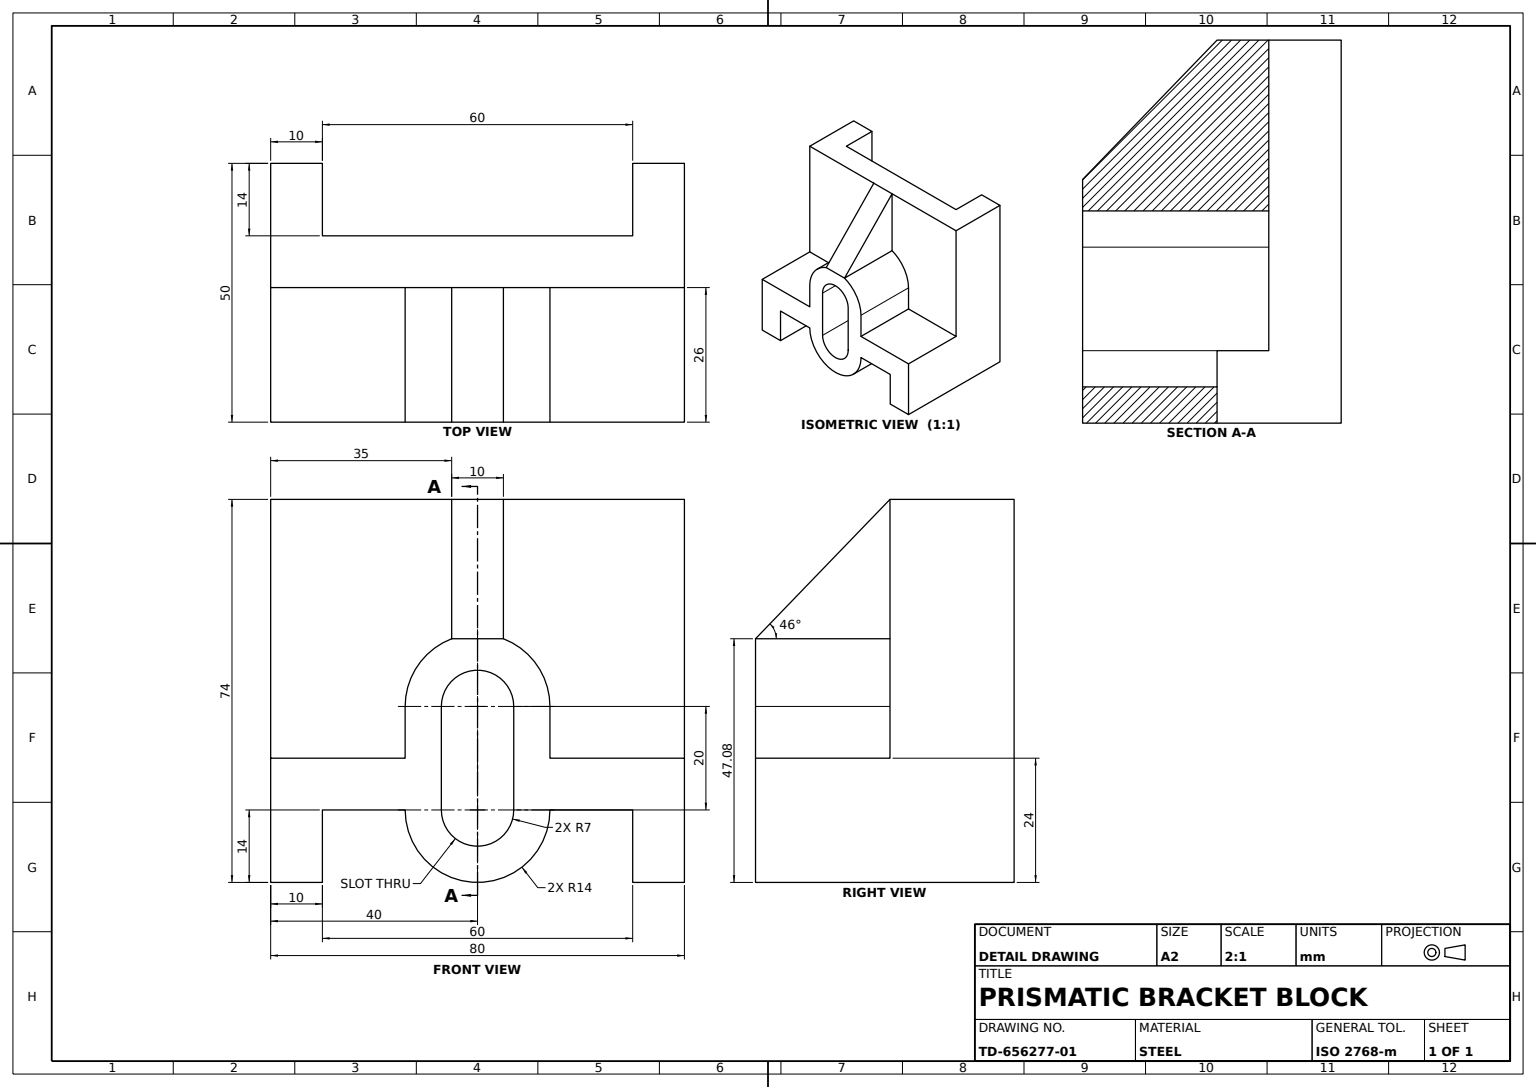
SolidWorks part; units mm, degrees
material "Plain Carbon Steel"
ref_plane "Front Plane" through (0, 0, 0) normal (0, 0, 1) x (1, 0, 0)
ref_plane "Top Plane" through (0, 0, 0) normal (0, 1, 0) x (1, 0, 0)
ref_plane "Right Plane" through (0, 0, 0) normal (1, 0, 0) x (0, 0, -1)
sketch "Base Profile Sketch" plane through (0, 0, 0) normal (0, 0, 1) x (1, 0, 0)
  line L0 (0, 0) -> (40, 0)
  line L1 (40, 0) -> (80, 0)
  line L2 (80, 0) -> (80, -24)
  line L3 (80, -24) -> (70, -24)
  line L4 (70, -24) -> (70, -10)
  line L5 (70, -10) -> (10, -10)
  line L6 (10, -10) -> (10, -24)
  line L7 (10, -24) -> (0, -24)
  line L8 (0, -24) -> (0, 0)
  dimension "D1" = 24
  dimension "D2" = 10
  dimension "D3" = 14
  dimension "D4" = 60
  dimension "D5" = 10
  dimension "D6" = 40
  dimension "D7" = 24
extrude "Base Body" add sketch "Base Profile Sketch" against normal blind 50
sketch "Back Wall Sketch" plane through (0, 0, 0) normal (0, 1, 0) x (1, 0, 0)
  line L0 (80, 50) -> (80, 0) construction
  line L1 (0, 50) -> (80, 50)
  line L2 (0, 50) -> (0, 26)
  line L3 (0, 26) -> (80, 26)
  line L4 (80, 50) -> (80, 26)
  dimension "D1" = 24
extrude "Back Wall" add sketch "Back Wall Sketch" along normal blind 50
sketch "Wall Notch Sketch" plane through (0, 50, 0) normal (0, 1, 0) x (1, 0, 0)
  line L0 (80, 50) -> (0, 50) construction
  line L1 (10, 50) -> (70, 50)
  line L2 (10, 50) -> (10, 36)
  line L3 (10, 36) -> (70, 36)
  line L4 (70, 50) -> (70, 36)
  dimension "D1" = 60
  dimension "D2" = 10
  dimension "D3" = 14
extrude "Wall Notch Cut" cut sketch "Wall Notch Sketch" against normal through all
sketch "Slot Boss Sketch" plane through (0, 0, 0) normal (0, 0, 1) x (1, 0, 0)
  line L0 (10, -10) -> (70, -10) construction
  line L1 (26, 10) -> (26, -10)
  line L2 (54, 10) -> (54, -10)
  arc A0 (54, 10) -> (26, 10) centre (40, 10) ccw
  arc A1 (26, -10) -> (54, -10) centre (40, -10) ccw
  dimension "D1" = 28
  dimension "D2" = 28
  dimension "D3" = 40
  dimension "D4" = 40
  dimension "D5" = 20
  dimension "D6" = 14
  dimension "D7" = 26
  dimension "D8" = 10
extrude "Slot Boss" add sketch "Slot Boss Sketch" against normal blind 26
sketch "Slot Sketch" plane through (0, 0, 0) normal (0, 0, 1) x (1, 0, 0)
  line L0 (33, -10) -> (33, 10)
  line L1 (47, -10) -> (47, 10)
  arc A0 (47, 10) -> (33, 10) centre (40, 10) ccw
  arc A1 (33, -10) -> (47, -10) centre (40, -10) ccw
  dimension "D1" = 14
  dimension "D2" = 14
  dimension "D3" = 33
  dimension "D4" = 47
extrude "Slot Cut 14mm" cut sketch "Slot Sketch" against normal through all
sketch "Rib Sketch" plane through (0, 0, -26) normal (0, 0, 1) x (1, 0, 0)
  line L0 (0, 50) -> (80, 50) construction
  line L1 (35, 50) -> (45, 50)
  line L2 (35, 50) -> (35, 23)
  line L3 (35, 23) -> (45, 23)
  line L4 (45, 50) -> (45, 23)
  line L5 (40, -17) -> (40, -10) construction
  arc A0 (33, -10) -> (47, -10) centre (40, -10) ccw construction
  dimension "D1" = 5
  dimension "D2" = 10
  dimension "D3" = 27
extrude "Reinforcing Rib" add sketch "Rib Sketch" along normal blind 26
sketch "Trim Line Sketch" plane through (35, 0, 0) normal (-1, 0, 0) x (0, 0, 1)
  line L0 (-26, 50) -> (0, 23.0767)
extrude "Trim Cut" cut sketch "Trim Line Sketch" against normal blind 26 and the other way through all
